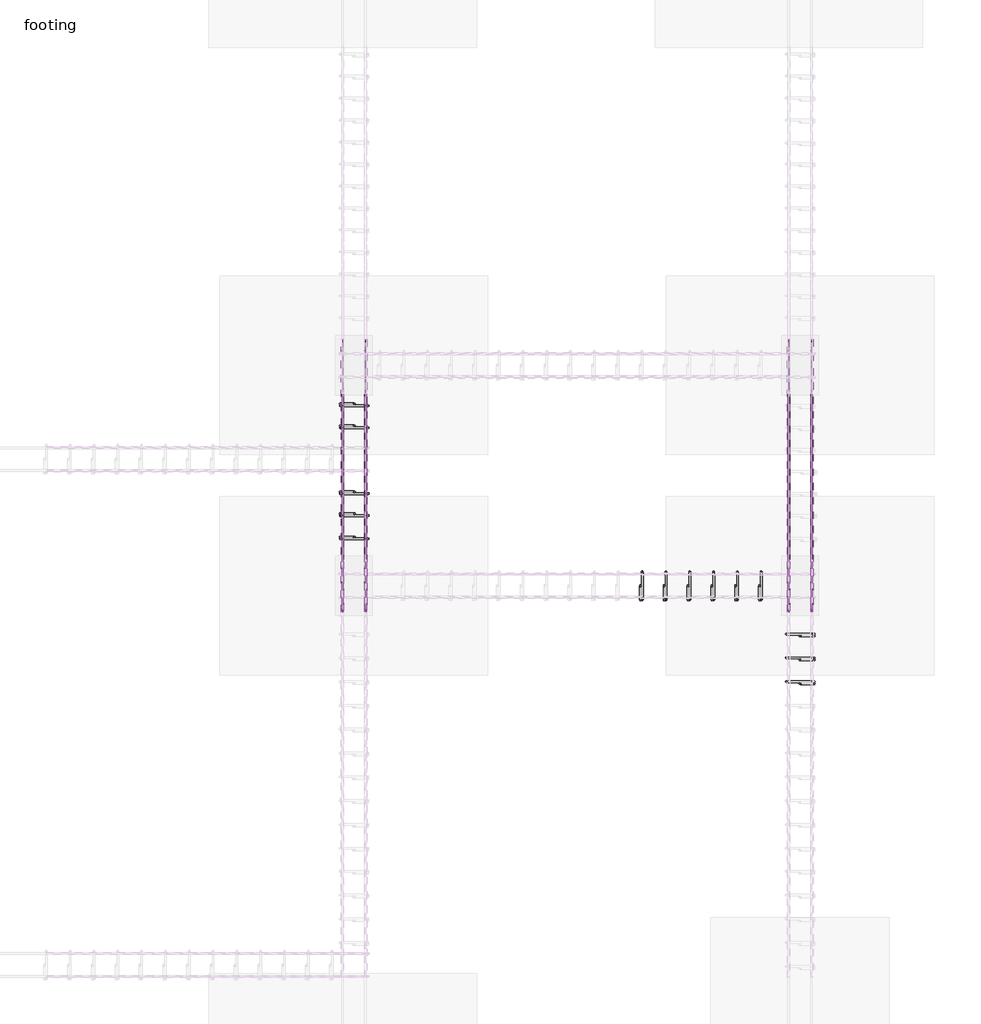
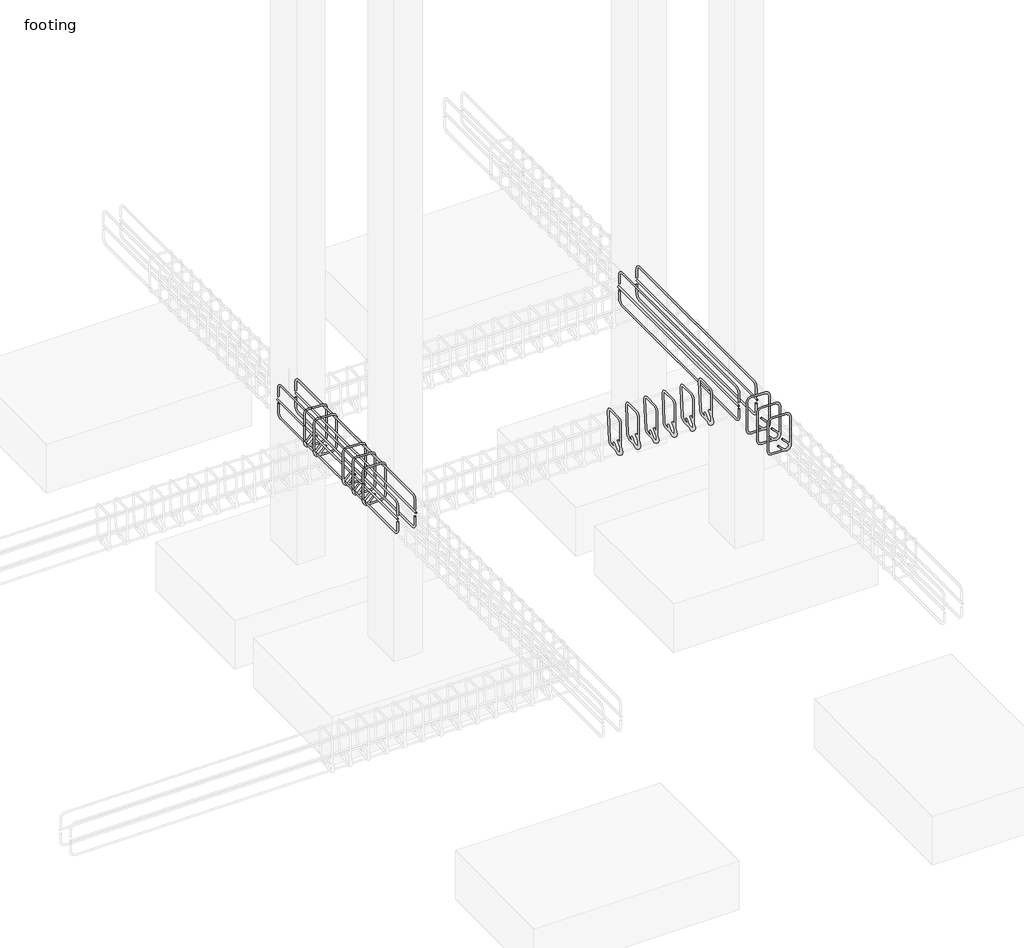
# One storey, part 14 of 21: 26 reinforcing bars.
"""IFC4 building model written with IfcOpenShell, lengths in millimetres."""

from ifc_helpers import new_model, si_unit, point, frame, origin, place, context, project, spatial, polyline, circle_curve, trimmed, segment, composite_curve, element, save
from ifc_brep_helpers import swept_disk

model = new_model("IFC4")

# Units and contexts
model_context = context("Model", 3, world=origin())
ifc_project = project(units=[si_unit("LENGTHUNIT", "METRE", prefix="MILLI")], contexts=[model_context])

# Site, building, storey
site = spatial("IfcSite", under=ifc_project)
building = spatial("IfcBuilding", under=site)
storey = spatial("IfcBuildingStorey", under=building, Name="footing", Elevation=-1524.0)

# Reinforcing bars
placement = place(None, origin())
element("IfcReinforcingBar", 1, at=placement, inside=storey, context=model_context, shape_type="SolidModel", body=[
    swept_disk(composite_curve([segment(polyline([(-5910.0883428, 6708.6887132, -310.8825168), (-5910.0883428, 6653.8237147, -365.7475153)]), True, "CONTINUOUS"), segment(trimmed(circle_curve(frame((-5910.0883428, 6631.3730744, -343.296875), z_axis=(-1.0, 0.0, 0.0), x_axis=(0.0, 22.450640299999577, -22.450640299999975)), 31.75), [point((-5910.0883428, 6653.8237147, -365.7475153))], [point((-5910.0883428, 6599.6230744, -343.296875))], True, "CARTESIAN"), True, "CONTINUOUS"), segment(polyline([(-5910.0883428, 6599.6230744, -343.296875), (-5910.0883428, 6599.6230744, -63.103125)]), True, "CONTINUOUS"), segment(trimmed(circle_curve(frame((-5910.0883428, 6631.3730744, -63.103125), z_axis=(-1.0, 0.0, 0.0), x_axis=(0.0, -31.75, 0.0)), 31.75), [point((-5910.0883428, 6599.6230744, -63.103125))], [point((-5910.0883428, 6631.3730744, -31.353125))], True, "CARTESIAN"), True, "CONTINUOUS"), segment(polyline([(-5910.0883428, 6631.3730744, -31.353125), (-5910.0883428, 6759.1668244, -31.353125)]), True, "CONTINUOUS"), segment(trimmed(circle_curve(frame((-5908.9159328, 6759.1668244, -63.0814712), z_axis=(-0.9993179916193466, 0.0, -0.03692629992126919), x_axis=(-1.1724100000001272, 0.0, 31.728346200000004)), 31.75), [point((-5910.0883428, 6759.1668244, -31.353125))], [point((-5908.9159328, 6790.9168244, -63.0814712))], True, "CARTESIAN"), True, "CONTINUOUS"), segment(polyline([(-5908.9159328, 6790.9168244, -63.0814712), (-5898.5607528, 6790.9168244, -343.3185288)]), True, "CONTINUOUS"), segment(trimmed(circle_curve(frame((-5898.5607528, 6759.1668244, -343.3185288), z_axis=(-0.9993179916193466, 0.0, -0.03692629992126919), x_axis=(0.0, 31.75, 0.0)), 31.75), [point((-5898.5607528, 6790.9168244, -343.3185288))], [point((-5897.3883428, 6759.1668244, -375.046875))], True, "CARTESIAN"), True, "CONTINUOUS"), segment(polyline([(-5897.3883428, 6759.1668244, -375.046875), (-5897.3883428, 6631.3730744, -375.046875)]), True, "CONTINUOUS"), segment(trimmed(circle_curve(frame((-5897.3883428, 6631.3730744, -343.296875), z_axis=(-1.0, 0.0, 0.0), x_axis=(0.0, 0.0, -31.75)), 31.75), [point((-5897.3883428, 6631.3730744, -375.046875))], [point((-5897.3883428, 6608.9224341, -320.8462347))], True, "CARTESIAN"), True, "CONTINUOUS"), segment(polyline([(-5897.3883428, 6608.9224341, -320.8462347), (-5897.3883428, 6663.7874326, -265.9812362)]), True, "CONTINUOUS")], self_intersect=False), 6.35),
])
element("IfcReinforcingBar", 2, at=placement, inside=storey, context=model_context, shape_type="SolidModel", body=[
    swept_disk(composite_curve([segment(polyline([(-5747.3883428, 6708.6887132, -310.8825168), (-5747.3883428, 6653.8237147, -365.7475153)]), True, "CONTINUOUS"), segment(trimmed(circle_curve(frame((-5747.3883428, 6631.3730744, -343.296875), z_axis=(-1.0, 0.0, 0.0), x_axis=(0.0, 22.450640299999577, -22.450640299999975)), 31.75), [point((-5747.3883428, 6653.8237147, -365.7475153))], [point((-5747.3883428, 6599.6230744, -343.296875))], True, "CARTESIAN"), True, "CONTINUOUS"), segment(polyline([(-5747.3883428, 6599.6230744, -343.296875), (-5747.3883428, 6599.6230744, -63.103125)]), True, "CONTINUOUS"), segment(trimmed(circle_curve(frame((-5747.3883428, 6631.3730744, -63.103125), z_axis=(-1.0, 0.0, 0.0), x_axis=(0.0, -31.75, 0.0)), 31.75), [point((-5747.3883428, 6599.6230744, -63.103125))], [point((-5747.3883428, 6631.3730744, -31.353125))], True, "CARTESIAN"), True, "CONTINUOUS"), segment(polyline([(-5747.3883428, 6631.3730744, -31.353125), (-5747.3883428, 6759.1668244, -31.353125)]), True, "CONTINUOUS"), segment(trimmed(circle_curve(frame((-5746.2159328, 6759.1668244, -63.0814712), z_axis=(-0.9993179916193466, 0.0, -0.03692629992126919), x_axis=(-1.1724100000001272, 0.0, 31.728346200000004)), 31.75), [point((-5747.3883428, 6759.1668244, -31.353125))], [point((-5746.2159328, 6790.9168244, -63.0814712))], True, "CARTESIAN"), True, "CONTINUOUS"), segment(polyline([(-5746.2159328, 6790.9168244, -63.0814712), (-5735.8607528, 6790.9168244, -343.3185288)]), True, "CONTINUOUS"), segment(trimmed(circle_curve(frame((-5735.8607528, 6759.1668244, -343.3185288), z_axis=(-0.9993179916193466, 0.0, -0.03692629992126919), x_axis=(0.0, 31.75, 0.0)), 31.75), [point((-5735.8607528, 6790.9168244, -343.3185288))], [point((-5734.6883428, 6759.1668244, -375.046875))], True, "CARTESIAN"), True, "CONTINUOUS"), segment(polyline([(-5734.6883428, 6759.1668244, -375.046875), (-5734.6883428, 6631.3730744, -375.046875)]), True, "CONTINUOUS"), segment(trimmed(circle_curve(frame((-5734.6883428, 6631.3730744, -343.296875), z_axis=(-1.0, 0.0, 0.0), x_axis=(0.0, 0.0, -31.75)), 31.75), [point((-5734.6883428, 6631.3730744, -375.046875))], [point((-5734.6883428, 6608.9224341, -320.8462347))], True, "CARTESIAN"), True, "CONTINUOUS"), segment(polyline([(-5734.6883428, 6608.9224341, -320.8462347), (-5734.6883428, 6663.7874326, -265.9812362)]), True, "CONTINUOUS")], self_intersect=False), 6.35),
])
element("IfcReinforcingBar", 3, at=placement, inside=storey, context=model_context, shape_type="SolidModel", body=[
    swept_disk(composite_curve([segment(polyline([(-5584.6883428, 6708.6887132, -310.8825168), (-5584.6883428, 6653.8237147, -365.7475153)]), True, "CONTINUOUS"), segment(trimmed(circle_curve(frame((-5584.6883428, 6631.3730744, -343.296875), z_axis=(-1.0, 0.0, 0.0), x_axis=(0.0, 22.450640299999577, -22.450640299999975)), 31.75), [point((-5584.6883428, 6653.8237147, -365.7475153))], [point((-5584.6883428, 6599.6230744, -343.296875))], True, "CARTESIAN"), True, "CONTINUOUS"), segment(polyline([(-5584.6883428, 6599.6230744, -343.296875), (-5584.6883428, 6599.6230744, -63.103125)]), True, "CONTINUOUS"), segment(trimmed(circle_curve(frame((-5584.6883428, 6631.3730744, -63.103125), z_axis=(-1.0, 0.0, 0.0), x_axis=(0.0, -31.75, 0.0)), 31.75), [point((-5584.6883428, 6599.6230744, -63.103125))], [point((-5584.6883428, 6631.3730744, -31.353125))], True, "CARTESIAN"), True, "CONTINUOUS"), segment(polyline([(-5584.6883428, 6631.3730744, -31.353125), (-5584.6883428, 6759.1668244, -31.353125)]), True, "CONTINUOUS"), segment(trimmed(circle_curve(frame((-5583.5159328, 6759.1668244, -63.0814712), z_axis=(-0.9993179916193466, 0.0, -0.03692629992126919), x_axis=(-1.1724100000001272, 0.0, 31.728346200000004)), 31.75), [point((-5584.6883428, 6759.1668244, -31.353125))], [point((-5583.5159328, 6790.9168244, -63.0814712))], True, "CARTESIAN"), True, "CONTINUOUS"), segment(polyline([(-5583.5159328, 6790.9168244, -63.0814712), (-5573.1607528, 6790.9168244, -343.3185288)]), True, "CONTINUOUS"), segment(trimmed(circle_curve(frame((-5573.1607528, 6759.1668244, -343.3185288), z_axis=(-0.9993179916193466, 0.0, -0.03692629992126919), x_axis=(0.0, 31.75, 0.0)), 31.75), [point((-5573.1607528, 6790.9168244, -343.3185288))], [point((-5571.9883428, 6759.1668244, -375.046875))], True, "CARTESIAN"), True, "CONTINUOUS"), segment(polyline([(-5571.9883428, 6759.1668244, -375.046875), (-5571.9883428, 6631.3730744, -375.046875)]), True, "CONTINUOUS"), segment(trimmed(circle_curve(frame((-5571.9883428, 6631.3730744, -343.296875), z_axis=(-1.0, 0.0, 0.0), x_axis=(0.0, 0.0, -31.75)), 31.75), [point((-5571.9883428, 6631.3730744, -375.046875))], [point((-5571.9883428, 6608.9224341, -320.8462347))], True, "CARTESIAN"), True, "CONTINUOUS"), segment(polyline([(-5571.9883428, 6608.9224341, -320.8462347), (-5571.9883428, 6663.7874326, -265.9812362)]), True, "CONTINUOUS")], self_intersect=False), 6.35),
])
element("IfcReinforcingBar", 4, at=placement, inside=storey, context=model_context, shape_type="SolidModel", body=[
    swept_disk(composite_curve([segment(polyline([(-5421.9883428, 6708.6887132, -310.8825168), (-5421.9883428, 6653.8237147, -365.7475153)]), True, "CONTINUOUS"), segment(trimmed(circle_curve(frame((-5421.9883428, 6631.3730744, -343.296875), z_axis=(-1.0, 0.0, 0.0), x_axis=(0.0, 22.450640299999577, -22.450640299999975)), 31.75), [point((-5421.9883428, 6653.8237147, -365.7475153))], [point((-5421.9883428, 6599.6230744, -343.296875))], True, "CARTESIAN"), True, "CONTINUOUS"), segment(polyline([(-5421.9883428, 6599.6230744, -343.296875), (-5421.9883428, 6599.6230744, -63.103125)]), True, "CONTINUOUS"), segment(trimmed(circle_curve(frame((-5421.9883428, 6631.3730744, -63.103125), z_axis=(-1.0, 0.0, 0.0), x_axis=(0.0, -31.75, 0.0)), 31.75), [point((-5421.9883428, 6599.6230744, -63.103125))], [point((-5421.9883428, 6631.3730744, -31.353125))], True, "CARTESIAN"), True, "CONTINUOUS"), segment(polyline([(-5421.9883428, 6631.3730744, -31.353125), (-5421.9883428, 6759.1668244, -31.353125)]), True, "CONTINUOUS"), segment(trimmed(circle_curve(frame((-5420.8159328, 6759.1668244, -63.0814712), z_axis=(-0.9993179916193466, 0.0, -0.03692629992126919), x_axis=(-1.1724100000001272, 0.0, 31.728346200000004)), 31.75), [point((-5421.9883428, 6759.1668244, -31.353125))], [point((-5420.8159328, 6790.9168244, -63.0814712))], True, "CARTESIAN"), True, "CONTINUOUS"), segment(polyline([(-5420.8159328, 6790.9168244, -63.0814712), (-5410.4607528, 6790.9168244, -343.3185288)]), True, "CONTINUOUS"), segment(trimmed(circle_curve(frame((-5410.4607528, 6759.1668244, -343.3185288), z_axis=(-0.9993179916193466, 0.0, -0.03692629992126919), x_axis=(0.0, 31.75, 0.0)), 31.75), [point((-5410.4607528, 6790.9168244, -343.3185288))], [point((-5409.2883428, 6759.1668244, -375.046875))], True, "CARTESIAN"), True, "CONTINUOUS"), segment(polyline([(-5409.2883428, 6759.1668244, -375.046875), (-5409.2883428, 6631.3730744, -375.046875)]), True, "CONTINUOUS"), segment(trimmed(circle_curve(frame((-5409.2883428, 6631.3730744, -343.296875), z_axis=(-1.0, 0.0, 0.0), x_axis=(0.0, 0.0, -31.75)), 31.75), [point((-5409.2883428, 6631.3730744, -375.046875))], [point((-5409.2883428, 6608.9224341, -320.8462347))], True, "CARTESIAN"), True, "CONTINUOUS"), segment(polyline([(-5409.2883428, 6608.9224341, -320.8462347), (-5409.2883428, 6663.7874326, -265.9812362)]), True, "CONTINUOUS")], self_intersect=False), 6.35),
])
element("IfcReinforcingBar", 5, at=placement, inside=storey, context=model_context, shape_type="SolidModel", body=[
    swept_disk(composite_curve([segment(polyline([(-5259.2883428, 6708.6887132, -310.8825168), (-5259.2883428, 6653.8237147, -365.7475153)]), True, "CONTINUOUS"), segment(trimmed(circle_curve(frame((-5259.2883428, 6631.3730744, -343.296875), z_axis=(-1.0, 0.0, 0.0), x_axis=(0.0, 22.450640299999577, -22.450640299999975)), 31.75), [point((-5259.2883428, 6653.8237147, -365.7475153))], [point((-5259.2883428, 6599.6230744, -343.296875))], True, "CARTESIAN"), True, "CONTINUOUS"), segment(polyline([(-5259.2883428, 6599.6230744, -343.296875), (-5259.2883428, 6599.6230744, -63.103125)]), True, "CONTINUOUS"), segment(trimmed(circle_curve(frame((-5259.2883428, 6631.3730744, -63.103125), z_axis=(-1.0, 0.0, 0.0), x_axis=(0.0, -31.75, 0.0)), 31.75), [point((-5259.2883428, 6599.6230744, -63.103125))], [point((-5259.2883428, 6631.3730744, -31.353125))], True, "CARTESIAN"), True, "CONTINUOUS"), segment(polyline([(-5259.2883428, 6631.3730744, -31.353125), (-5259.2883428, 6759.1668244, -31.353125)]), True, "CONTINUOUS"), segment(trimmed(circle_curve(frame((-5258.1159328, 6759.1668244, -63.0814712), z_axis=(-0.9993179916193466, 0.0, -0.03692629992126919), x_axis=(-1.1724099999992177, 0.0, 31.728346200000004)), 31.75), [point((-5259.2883428, 6759.1668244, -31.353125))], [point((-5258.1159328, 6790.9168244, -63.0814712))], True, "CARTESIAN"), True, "CONTINUOUS"), segment(polyline([(-5258.1159328, 6790.9168244, -63.0814712), (-5247.7607528, 6790.9168244, -343.3185288)]), True, "CONTINUOUS"), segment(trimmed(circle_curve(frame((-5247.7607528, 6759.1668244, -343.3185288), z_axis=(-0.9993179916193466, 0.0, -0.03692629992126919), x_axis=(0.0, 31.75, 0.0)), 31.75), [point((-5247.7607528, 6790.9168244, -343.3185288))], [point((-5246.5883428, 6759.1668244, -375.046875))], True, "CARTESIAN"), True, "CONTINUOUS"), segment(polyline([(-5246.5883428, 6759.1668244, -375.046875), (-5246.5883428, 6631.3730744, -375.046875)]), True, "CONTINUOUS"), segment(trimmed(circle_curve(frame((-5246.5883428, 6631.3730744, -343.296875), z_axis=(-1.0, 0.0, 0.0), x_axis=(0.0, 0.0, -31.75)), 31.75), [point((-5246.5883428, 6631.3730744, -375.046875))], [point((-5246.5883428, 6608.9224341, -320.8462347))], True, "CARTESIAN"), True, "CONTINUOUS"), segment(polyline([(-5246.5883428, 6608.9224341, -320.8462347), (-5246.5883428, 6663.7874326, -265.9812362)]), True, "CONTINUOUS")], self_intersect=False), 6.35),
])
element("IfcReinforcingBar", 6, at=placement, inside=storey, context=model_context, shape_type="SolidModel", body=[
    swept_disk(composite_curve([segment(polyline([(-5096.5883428, 6708.6887132, -310.8825168), (-5096.5883428, 6653.8237147, -365.7475153)]), True, "CONTINUOUS"), segment(trimmed(circle_curve(frame((-5096.5883428, 6631.3730744, -343.296875), z_axis=(-1.0, 0.0, 0.0), x_axis=(0.0, 22.450640299999577, -22.450640299999975)), 31.75), [point((-5096.5883428, 6653.8237147, -365.7475153))], [point((-5096.5883428, 6599.6230744, -343.296875))], True, "CARTESIAN"), True, "CONTINUOUS"), segment(polyline([(-5096.5883428, 6599.6230744, -343.296875), (-5096.5883428, 6599.6230744, -63.103125)]), True, "CONTINUOUS"), segment(trimmed(circle_curve(frame((-5096.5883428, 6631.3730744, -63.103125), z_axis=(-1.0, 0.0, 0.0), x_axis=(0.0, -31.75, 0.0)), 31.75), [point((-5096.5883428, 6599.6230744, -63.103125))], [point((-5096.5883428, 6631.3730744, -31.353125))], True, "CARTESIAN"), True, "CONTINUOUS"), segment(polyline([(-5096.5883428, 6631.3730744, -31.353125), (-5096.5883428, 6759.1668244, -31.353125)]), True, "CONTINUOUS"), segment(trimmed(circle_curve(frame((-5095.4159328, 6759.1668244, -63.0814712), z_axis=(-0.9993179916193466, 0.0, -0.03692629992126919), x_axis=(-1.1724100000001272, 0.0, 31.728346200000004)), 31.75), [point((-5096.5883428, 6759.1668244, -31.353125))], [point((-5095.4159328, 6790.9168244, -63.0814712))], True, "CARTESIAN"), True, "CONTINUOUS"), segment(polyline([(-5095.4159328, 6790.9168244, -63.0814712), (-5085.0607528, 6790.9168244, -343.3185288)]), True, "CONTINUOUS"), segment(trimmed(circle_curve(frame((-5085.0607528, 6759.1668244, -343.3185288), z_axis=(-0.9993179916193466, 0.0, -0.03692629992126919), x_axis=(0.0, 31.75, 0.0)), 31.75), [point((-5085.0607528, 6790.9168244, -343.3185288))], [point((-5083.8883428, 6759.1668244, -375.046875))], True, "CARTESIAN"), True, "CONTINUOUS"), segment(polyline([(-5083.8883428, 6759.1668244, -375.046875), (-5083.8883428, 6631.3730744, -375.046875)]), True, "CONTINUOUS"), segment(trimmed(circle_curve(frame((-5083.8883428, 6631.3730744, -343.296875), z_axis=(-1.0, 0.0, 0.0), x_axis=(0.0, 0.0, -31.75)), 31.75), [point((-5083.8883428, 6631.3730744, -375.046875))], [point((-5083.8883428, 6608.9224341, -320.8462347))], True, "CARTESIAN"), True, "CONTINUOUS"), segment(polyline([(-5083.8883428, 6608.9224341, -320.8462347), (-5083.8883428, 6663.7874326, -265.9812362)]), True, "CONTINUOUS")], self_intersect=False), 6.35),
])
element("IfcReinforcingBar", 7, at=placement, inside=storey, context=model_context, shape_type="SolidModel", body=[
    swept_disk(composite_curve([segment(polyline([(-7897.6815591, 7925.2699494, -265.9812362), (-7952.5465576, 7925.2699494, -320.8462347)]), True, "CONTINUOUS"), segment(trimmed(circle_curve(frame((-7930.0959173, 7925.2699494, -343.296875), z_axis=(0.0, -1.0, 0.0), x_axis=(-22.450640299999577, 0.0, 22.450640299999975)), 31.75), [point((-7952.5465576, 7925.2699494, -320.8462347))], [point((-7930.0959173, 7925.2699494, -375.046875))], True, "CARTESIAN"), True, "CONTINUOUS"), segment(polyline([(-7930.0959173, 7925.2699494, -375.046875), (-7802.3021673, 7925.2699494, -375.046875)]), True, "CONTINUOUS"), segment(trimmed(circle_curve(frame((-7802.3021673, 7925.2699494, -343.296875), z_axis=(0.0, -1.0, 0.0), x_axis=(0.0, 0.0, -31.75)), 31.75), [point((-7802.3021673, 7925.2699494, -375.046875))], [point((-7770.5521673, 7925.2699494, -343.296875))], True, "CARTESIAN"), True, "CONTINUOUS"), segment(polyline([(-7770.5521673, 7925.2699494, -343.296875), (-7770.5521673, 7925.2699494, -63.103125)]), True, "CONTINUOUS"), segment(trimmed(circle_curve(frame((-7802.2324265, 7927.3732031, -63.103125), z_axis=(-0.06624421176864148, -0.9978034397651431, 0.0), x_axis=(31.680259199999455, -2.1032537000000957, 0.0)), 31.75), [point((-7770.5521673, 7925.2699494, -63.103125))], [point((-7802.2324265, 7927.3732031, -31.353125))], True, "CARTESIAN"), True, "CONTINUOUS"), segment(polyline([(-7802.2324265, 7927.3732031, -31.353125), (-7930.165658, 7935.8666957, -31.353125)]), True, "CONTINUOUS"), segment(trimmed(circle_curve(frame((-7930.165658, 7935.8666957, -63.103125), z_axis=(-0.06624421176864148, -0.9978034397651431, 0.0), x_axis=(0.0, 0.0, 31.75)), 31.75), [point((-7930.165658, 7935.8666957, -31.353125))], [point((-7961.8459173, 7937.9699494, -63.103125))], True, "CARTESIAN"), True, "CONTINUOUS"), segment(polyline([(-7961.8459173, 7937.9699494, -63.103125), (-7961.8459173, 7937.9699494, -343.296875)]), True, "CONTINUOUS"), segment(trimmed(circle_curve(frame((-7930.0959173, 7937.9699494, -343.296875), z_axis=(0.0, -1.0, 0.0), x_axis=(-31.75, 0.0, 0.0)), 31.75), [point((-7961.8459173, 7937.9699494, -343.296875))], [point((-7907.645277, 7937.9699494, -365.7475153))], True, "CARTESIAN"), True, "CONTINUOUS"), segment(polyline([(-7907.645277, 7937.9699494, -365.7475153), (-7852.7802785, 7937.9699494, -310.8825168)]), True, "CONTINUOUS")], self_intersect=False), 6.35),
])
element("IfcReinforcingBar", 8, at=placement, inside=storey, context=model_context, shape_type="SolidModel", body=[
    swept_disk(composite_curve([segment(polyline([(-7943.5663014, 8372.0668244, -170.2827408), (-7943.5663014, 8372.0668244, -94.0827408)]), True, "CONTINUOUS"), segment(trimmed(circle_curve(frame((-7943.5663014, 8327.6168244, -94.0827408), z_axis=(1.0, 0.0, 0.0), x_axis=(0.0, 44.45000000000073, 0.0)), 44.45), [point((-7943.5663014, 8372.0668244, -94.0827408))], [point((-7943.5663014, 8327.6168244, -49.6327408))], True, "CARTESIAN"), True, "CONTINUOUS"), segment(polyline([(-7943.5663014, 8327.6168244, -49.6327408), (-7943.5663014, 6567.8730744, -49.6327408)]), True, "CONTINUOUS"), segment(trimmed(circle_curve(frame((-7943.5663014, 6567.8730744, -94.0827408), z_axis=(1.0, 0.0, 0.0), x_axis=(0.0, 0.0, 44.449999999999996)), 44.45), [point((-7943.5663014, 6567.8730744, -49.6327408))], [point((-7943.5663014, 6523.4230744, -94.0827408))], True, "CARTESIAN"), True, "CONTINUOUS"), segment(polyline([(-7943.5663014, 6523.4230744, -94.0827408), (-7943.5663014, 6523.4230744, -170.2827408)]), True, "CONTINUOUS")], self_intersect=False), 6.35),
])
element("IfcReinforcingBar", 9, at=placement, inside=storey, context=model_context, shape_type="SolidModel", body=[
    swept_disk(composite_curve([segment(polyline([(-7788.8317831, 8372.0668244, -170.2827408), (-7788.8317831, 8372.0668244, -94.0827408)]), True, "CONTINUOUS"), segment(trimmed(circle_curve(frame((-7788.8317831, 8327.6168244, -94.0827408), z_axis=(1.0, 0.0, 0.0), x_axis=(0.0, 44.45000000000073, 0.0)), 44.45), [point((-7788.8317831, 8372.0668244, -94.0827408))], [point((-7788.8317831, 8327.6168244, -49.6327408))], True, "CARTESIAN"), True, "CONTINUOUS"), segment(polyline([(-7788.8317831, 8327.6168244, -49.6327408), (-7788.8317831, 6567.8730744, -49.6327408)]), True, "CONTINUOUS"), segment(trimmed(circle_curve(frame((-7788.8317831, 6567.8730744, -94.0827408), z_axis=(1.0, 0.0, 0.0), x_axis=(0.0, 0.0, 44.449999999999996)), 44.45), [point((-7788.8317831, 6567.8730744, -49.6327408))], [point((-7788.8317831, 6523.4230744, -94.0827408))], True, "CARTESIAN"), True, "CONTINUOUS"), segment(polyline([(-7788.8317831, 6523.4230744, -94.0827408), (-7788.8317831, 6523.4230744, -170.2827408)]), True, "CONTINUOUS")], self_intersect=False), 6.35),
])
element("IfcReinforcingBar", 10, at=placement, inside=storey, context=model_context, shape_type="SolidModel", body=[
    swept_disk(composite_curve([segment(polyline([(-7943.5663014, 8372.0668244, -236.1172592), (-7943.5663014, 8372.0668244, -312.3172592)]), True, "CONTINUOUS"), segment(trimmed(circle_curve(frame((-7943.5663014, 8327.6168244, -312.3172592), z_axis=(-1.0, 0.0, 0.0), x_axis=(0.0, 44.45000000000073, 0.0)), 44.45), [point((-7943.5663014, 8372.0668244, -312.3172592))], [point((-7943.5663014, 8327.6168244, -356.7672592))], True, "CARTESIAN"), True, "CONTINUOUS"), segment(polyline([(-7943.5663014, 8327.6168244, -356.7672592), (-7943.5663014, 6567.8730744, -356.7672592)]), True, "CONTINUOUS"), segment(trimmed(circle_curve(frame((-7943.5663014, 6567.8730744, -312.3172592), z_axis=(-1.0, 0.0, 0.0), x_axis=(0.0, 0.0, -44.44999999999999)), 44.45), [point((-7943.5663014, 6567.8730744, -356.7672592))], [point((-7943.5663014, 6523.4230744, -312.3172592))], True, "CARTESIAN"), True, "CONTINUOUS"), segment(polyline([(-7943.5663014, 6523.4230744, -312.3172592), (-7943.5663014, 6523.4230744, -236.1172592)]), True, "CONTINUOUS")], self_intersect=False), 6.35),
])
element("IfcReinforcingBar", 11, at=placement, inside=storey, context=model_context, shape_type="SolidModel", body=[
    swept_disk(composite_curve([segment(polyline([(-7788.8317831, 8372.0668244, -236.1172592), (-7788.8317831, 8372.0668244, -312.3172592)]), True, "CONTINUOUS"), segment(trimmed(circle_curve(frame((-7788.8317831, 8327.6168244, -312.3172592), z_axis=(-1.0, 0.0, 0.0), x_axis=(0.0, 44.45000000000073, 0.0)), 44.45), [point((-7788.8317831, 8372.0668244, -312.3172592))], [point((-7788.8317831, 8327.6168244, -356.7672592))], True, "CARTESIAN"), True, "CONTINUOUS"), segment(polyline([(-7788.8317831, 8327.6168244, -356.7672592), (-7788.8317831, 6567.8730744, -356.7672592)]), True, "CONTINUOUS"), segment(trimmed(circle_curve(frame((-7788.8317831, 6567.8730744, -312.3172592), z_axis=(-1.0, 0.0, 0.0), x_axis=(0.0, 0.0, -44.44999999999999)), 44.45), [point((-7788.8317831, 6567.8730744, -356.7672592))], [point((-7788.8317831, 6523.4230744, -312.3172592))], True, "CARTESIAN"), True, "CONTINUOUS"), segment(polyline([(-7788.8317831, 6523.4230744, -312.3172592), (-7788.8317831, 6523.4230744, -236.1172592)]), True, "CONTINUOUS")], self_intersect=False), 6.35),
])
element("IfcReinforcingBar", 12, at=placement, inside=storey, context=model_context, shape_type="SolidModel", body=[
    swept_disk(composite_curve([segment(polyline([(-7949.1459173, 8378.4168244, -203.2), (-7949.1459173, 6517.0730744, -203.2)]), True, "CONTINUOUS")], self_intersect=False), 6.35),
])
element("IfcReinforcingBar", 13, at=placement, inside=storey, context=model_context, shape_type="SolidModel", body=[
    swept_disk(composite_curve([segment(polyline([(-7783.2521673, 8378.4168244, -203.2), (-7783.2521673, 6517.0730744, -203.2)]), True, "CONTINUOUS")], self_intersect=False), 6.35),
])
element("IfcReinforcingBar", 14, at=placement, inside=storey, context=model_context, shape_type="SolidModel", body=[
    swept_disk(composite_curve([segment(polyline([(-7897.6815591, 7775.2699494, -265.9812362), (-7952.5465576, 7775.2699494, -320.8462347)]), True, "CONTINUOUS"), segment(trimmed(circle_curve(frame((-7930.0959173, 7775.2699494, -343.296875), z_axis=(0.0, -1.0, 0.0), x_axis=(-22.450640299999577, 0.0, 22.450640299999975)), 31.75), [point((-7952.5465576, 7775.2699494, -320.8462347))], [point((-7930.0959173, 7775.2699494, -375.046875))], True, "CARTESIAN"), True, "CONTINUOUS"), segment(polyline([(-7930.0959173, 7775.2699494, -375.046875), (-7802.3021673, 7775.2699494, -375.046875)]), True, "CONTINUOUS"), segment(trimmed(circle_curve(frame((-7802.3021673, 7775.2699494, -343.296875), z_axis=(0.0, -1.0, 0.0), x_axis=(0.0, 0.0, -31.75)), 31.75), [point((-7802.3021673, 7775.2699494, -375.046875))], [point((-7770.5521673, 7775.2699494, -343.296875))], True, "CARTESIAN"), True, "CONTINUOUS"), segment(polyline([(-7770.5521673, 7775.2699494, -343.296875), (-7770.5521673, 7775.2699494, -63.103125)]), True, "CONTINUOUS"), segment(trimmed(circle_curve(frame((-7802.2324265, 7777.3732031, -63.103125), z_axis=(-0.06624421176864148, -0.9978034397651431, 0.0), x_axis=(31.680259199999455, -2.1032537000000957, 0.0)), 31.75), [point((-7770.5521673, 7775.2699494, -63.103125))], [point((-7802.2324265, 7777.3732031, -31.353125))], True, "CARTESIAN"), True, "CONTINUOUS"), segment(polyline([(-7802.2324265, 7777.3732031, -31.353125), (-7930.165658, 7785.8666957, -31.353125)]), True, "CONTINUOUS"), segment(trimmed(circle_curve(frame((-7930.165658, 7785.8666957, -63.103125), z_axis=(-0.06624421176864148, -0.9978034397651431, 0.0), x_axis=(0.0, 0.0, 31.75)), 31.75), [point((-7930.165658, 7785.8666957, -31.353125))], [point((-7961.8459173, 7787.9699494, -63.103125))], True, "CARTESIAN"), True, "CONTINUOUS"), segment(polyline([(-7961.8459173, 7787.9699494, -63.103125), (-7961.8459173, 7787.9699494, -343.296875)]), True, "CONTINUOUS"), segment(trimmed(circle_curve(frame((-7930.0959173, 7787.9699494, -343.296875), z_axis=(0.0, -1.0, 0.0), x_axis=(-31.75, 0.0, 0.0)), 31.75), [point((-7961.8459173, 7787.9699494, -343.296875))], [point((-7907.645277, 7787.9699494, -365.7475153))], True, "CARTESIAN"), True, "CONTINUOUS"), segment(polyline([(-7907.645277, 7787.9699494, -365.7475153), (-7852.7802785, 7787.9699494, -310.8825168)]), True, "CONTINUOUS")], self_intersect=False), 6.35),
])
element("IfcReinforcingBar", 15, at=placement, inside=storey, context=model_context, shape_type="SolidModel", body=[
    swept_disk(composite_curve([segment(polyline([(-7897.6815591, 7325.2699494, -265.9812362), (-7952.5465576, 7325.2699494, -320.8462347)]), True, "CONTINUOUS"), segment(trimmed(circle_curve(frame((-7930.0959173, 7325.2699494, -343.296875), z_axis=(0.0, -1.0, 0.0), x_axis=(-22.450640299999577, 0.0, 22.450640299999975)), 31.75), [point((-7952.5465576, 7325.2699494, -320.8462347))], [point((-7930.0959173, 7325.2699494, -375.046875))], True, "CARTESIAN"), True, "CONTINUOUS"), segment(polyline([(-7930.0959173, 7325.2699494, -375.046875), (-7802.3021673, 7325.2699494, -375.046875)]), True, "CONTINUOUS"), segment(trimmed(circle_curve(frame((-7802.3021673, 7325.2699494, -343.296875), z_axis=(0.0, -1.0, 0.0), x_axis=(0.0, 0.0, -31.75)), 31.75), [point((-7802.3021673, 7325.2699494, -375.046875))], [point((-7770.5521673, 7325.2699494, -343.296875))], True, "CARTESIAN"), True, "CONTINUOUS"), segment(polyline([(-7770.5521673, 7325.2699494, -343.296875), (-7770.5521673, 7325.2699494, -63.103125)]), True, "CONTINUOUS"), segment(trimmed(circle_curve(frame((-7802.2324265, 7327.3732031, -63.103125), z_axis=(-0.06624421176864148, -0.9978034397651431, 0.0), x_axis=(31.680259199999455, -2.1032537000000957, 0.0)), 31.75), [point((-7770.5521673, 7325.2699494, -63.103125))], [point((-7802.2324265, 7327.3732031, -31.353125))], True, "CARTESIAN"), True, "CONTINUOUS"), segment(polyline([(-7802.2324265, 7327.3732031, -31.353125), (-7930.165658, 7335.8666957, -31.353125)]), True, "CONTINUOUS"), segment(trimmed(circle_curve(frame((-7930.165658, 7335.8666957, -63.103125), z_axis=(-0.06624421176864148, -0.9978034397651431, 0.0), x_axis=(0.0, 0.0, 31.75)), 31.75), [point((-7930.165658, 7335.8666957, -31.353125))], [point((-7961.8459173, 7337.9699494, -63.103125))], True, "CARTESIAN"), True, "CONTINUOUS"), segment(polyline([(-7961.8459173, 7337.9699494, -63.103125), (-7961.8459173, 7337.9699494, -343.296875)]), True, "CONTINUOUS"), segment(trimmed(circle_curve(frame((-7930.0959173, 7337.9699494, -343.296875), z_axis=(0.0, -1.0, 0.0), x_axis=(-31.75, 0.0, 0.0)), 31.75), [point((-7961.8459173, 7337.9699494, -343.296875))], [point((-7907.645277, 7337.9699494, -365.7475153))], True, "CARTESIAN"), True, "CONTINUOUS"), segment(polyline([(-7907.645277, 7337.9699494, -365.7475153), (-7852.7802785, 7337.9699494, -310.8825168)]), True, "CONTINUOUS")], self_intersect=False), 6.35),
])
element("IfcReinforcingBar", 16, at=placement, inside=storey, context=model_context, shape_type="SolidModel", body=[
    swept_disk(composite_curve([segment(polyline([(-7897.6815591, 7175.2699494, -265.9812362), (-7952.5465576, 7175.2699494, -320.8462347)]), True, "CONTINUOUS"), segment(trimmed(circle_curve(frame((-7930.0959173, 7175.2699494, -343.296875), z_axis=(0.0, -1.0, 0.0), x_axis=(-22.450640299999577, 0.0, 22.450640299999975)), 31.75), [point((-7952.5465576, 7175.2699494, -320.8462347))], [point((-7930.0959173, 7175.2699494, -375.046875))], True, "CARTESIAN"), True, "CONTINUOUS"), segment(polyline([(-7930.0959173, 7175.2699494, -375.046875), (-7802.3021673, 7175.2699494, -375.046875)]), True, "CONTINUOUS"), segment(trimmed(circle_curve(frame((-7802.3021673, 7175.2699494, -343.296875), z_axis=(0.0, -1.0, 0.0), x_axis=(0.0, 0.0, -31.75)), 31.75), [point((-7802.3021673, 7175.2699494, -375.046875))], [point((-7770.5521673, 7175.2699494, -343.296875))], True, "CARTESIAN"), True, "CONTINUOUS"), segment(polyline([(-7770.5521673, 7175.2699494, -343.296875), (-7770.5521673, 7175.2699494, -63.103125)]), True, "CONTINUOUS"), segment(trimmed(circle_curve(frame((-7802.2324265, 7177.3732031, -63.103125), z_axis=(-0.06624421176864148, -0.9978034397651431, 0.0), x_axis=(31.680259199999455, -2.1032537000000957, 0.0)), 31.75), [point((-7770.5521673, 7175.2699494, -63.103125))], [point((-7802.2324265, 7177.3732031, -31.353125))], True, "CARTESIAN"), True, "CONTINUOUS"), segment(polyline([(-7802.2324265, 7177.3732031, -31.353125), (-7930.165658, 7185.8666957, -31.353125)]), True, "CONTINUOUS"), segment(trimmed(circle_curve(frame((-7930.165658, 7185.8666957, -63.103125), z_axis=(-0.06624421176864148, -0.9978034397651431, 0.0), x_axis=(0.0, 0.0, 31.75)), 31.75), [point((-7930.165658, 7185.8666957, -31.353125))], [point((-7961.8459173, 7187.9699494, -63.103125))], True, "CARTESIAN"), True, "CONTINUOUS"), segment(polyline([(-7961.8459173, 7187.9699494, -63.103125), (-7961.8459173, 7187.9699494, -343.296875)]), True, "CONTINUOUS"), segment(trimmed(circle_curve(frame((-7930.0959173, 7187.9699494, -343.296875), z_axis=(0.0, -1.0, 0.0), x_axis=(-31.75, 0.0, 0.0)), 31.75), [point((-7961.8459173, 7187.9699494, -343.296875))], [point((-7907.645277, 7187.9699494, -365.7475153))], True, "CARTESIAN"), True, "CONTINUOUS"), segment(polyline([(-7907.645277, 7187.9699494, -365.7475153), (-7852.7802785, 7187.9699494, -310.8825168)]), True, "CONTINUOUS")], self_intersect=False), 6.35),
])
element("IfcReinforcingBar", 17, at=placement, inside=storey, context=model_context, shape_type="SolidModel", body=[
    swept_disk(composite_curve([segment(polyline([(-7897.6815591, 7016.6456073, -265.9812362), (-7952.5465576, 7016.6456073, -320.8462347)]), True, "CONTINUOUS"), segment(trimmed(circle_curve(frame((-7930.0959173, 7016.6456073, -343.296875), z_axis=(0.0, -1.0, 0.0), x_axis=(-22.450640299999577, 0.0, 22.450640299999975)), 31.75), [point((-7952.5465576, 7016.6456073, -320.8462347))], [point((-7930.0959173, 7016.6456073, -375.046875))], True, "CARTESIAN"), True, "CONTINUOUS"), segment(polyline([(-7930.0959173, 7016.6456073, -375.046875), (-7802.3021673, 7016.6456073, -375.046875)]), True, "CONTINUOUS"), segment(trimmed(circle_curve(frame((-7802.3021673, 7016.6456073, -343.296875), z_axis=(0.0, -1.0, 0.0), x_axis=(0.0, 0.0, -31.75)), 31.75), [point((-7802.3021673, 7016.6456073, -375.046875))], [point((-7770.5521673, 7016.6456073, -343.296875))], True, "CARTESIAN"), True, "CONTINUOUS"), segment(polyline([(-7770.5521673, 7016.6456073, -343.296875), (-7770.5521673, 7016.6456073, -63.103125)]), True, "CONTINUOUS"), segment(trimmed(circle_curve(frame((-7802.2324265, 7018.748861, -63.103125), z_axis=(-0.06624421176864148, -0.9978034397651431, 0.0), x_axis=(31.680259199999455, -2.1032537000000957, 0.0)), 31.75), [point((-7770.5521673, 7016.6456073, -63.103125))], [point((-7802.2324265, 7018.748861, -31.353125))], True, "CARTESIAN"), True, "CONTINUOUS"), segment(polyline([(-7802.2324265, 7018.748861, -31.353125), (-7930.165658, 7027.2423536, -31.353125)]), True, "CONTINUOUS"), segment(trimmed(circle_curve(frame((-7930.165658, 7027.2423536, -63.103125), z_axis=(-0.06624421176864148, -0.9978034397651431, 0.0), x_axis=(0.0, 0.0, 31.75)), 31.75), [point((-7930.165658, 7027.2423536, -31.353125))], [point((-7961.8459173, 7029.3456073, -63.103125))], True, "CARTESIAN"), True, "CONTINUOUS"), segment(polyline([(-7961.8459173, 7029.3456073, -63.103125), (-7961.8459173, 7029.3456073, -343.296875)]), True, "CONTINUOUS"), segment(trimmed(circle_curve(frame((-7930.0959173, 7029.3456073, -343.296875), z_axis=(0.0, -1.0, 0.0), x_axis=(-31.75, 0.0, 0.0)), 31.75), [point((-7961.8459173, 7029.3456073, -343.296875))], [point((-7907.645277, 7029.3456073, -365.7475153))], True, "CARTESIAN"), True, "CONTINUOUS"), segment(polyline([(-7907.645277, 7029.3456073, -365.7475153), (-7852.7802785, 7029.3456073, -310.8825168)]), True, "CONTINUOUS")], self_intersect=False), 6.35),
])
element("IfcReinforcingBar", 18, at=placement, inside=storey, context=model_context, shape_type="SolidModel", body=[
    swept_disk(composite_curve([segment(polyline([(-4786.7165254, 6040.4456073, -265.9812362), (-4731.851527, 6040.4456073, -320.8462347)]), True, "CONTINUOUS"), segment(trimmed(circle_curve(frame((-4754.3021673, 6040.4456073, -343.296875), z_axis=(0.0, 1.0, 0.0), x_axis=(22.450640300000487, 0.0, 22.450640299999975)), 31.75), [point((-4731.851527, 6040.4456073, -320.8462347))], [point((-4754.3021673, 6040.4456073, -375.046875))], True, "CARTESIAN"), True, "CONTINUOUS"), segment(polyline([(-4754.3021673, 6040.4456073, -375.046875), (-4882.0959173, 6040.4456073, -375.046875)]), True, "CONTINUOUS"), segment(trimmed(circle_curve(frame((-4882.0959173, 6040.4456073, -343.296875), z_axis=(0.0, 1.0, 0.0), x_axis=(0.0, 0.0, -31.75)), 31.75), [point((-4882.0959173, 6040.4456073, -375.046875))], [point((-4913.8459173, 6040.4456073, -343.296875))], True, "CARTESIAN"), True, "CONTINUOUS"), segment(polyline([(-4913.8459173, 6040.4456073, -343.296875), (-4913.8459173, 6040.4456073, -63.103125)]), True, "CONTINUOUS"), segment(trimmed(circle_curve(frame((-4882.165658, 6038.3423536, -63.103125), z_axis=(0.0662442117686417, 0.9978034397651431, 0.0), x_axis=(-31.680259300000216, 2.1032537000000957, 0.0)), 31.75), [point((-4913.8459173, 6040.4456073, -63.103125))], [point((-4882.165658, 6038.3423536, -31.353125))], True, "CARTESIAN"), True, "CONTINUOUS"), segment(polyline([(-4882.165658, 6038.3423536, -31.353125), (-4754.2324265, 6029.848861, -31.353125)]), True, "CONTINUOUS"), segment(trimmed(circle_curve(frame((-4754.2324265, 6029.848861, -63.103125), z_axis=(0.06624421176864169, 0.997803439765143, 0.0), x_axis=(0.0, 0.0, 31.75)), 31.75), [point((-4754.2324265, 6029.848861, -31.353125))], [point((-4722.5521673, 6027.7456073, -63.103125))], True, "CARTESIAN"), True, "CONTINUOUS"), segment(polyline([(-4722.5521673, 6027.7456073, -63.103125), (-4722.5521673, 6027.7456073, -343.296875)]), True, "CONTINUOUS"), segment(trimmed(circle_curve(frame((-4754.3021673, 6027.7456073, -343.296875), z_axis=(0.0, 1.0, 0.0), x_axis=(31.75, 0.0, 0.0)), 31.75), [point((-4722.5521673, 6027.7456073, -343.296875))], [point((-4776.7528076, 6027.7456073, -365.7475153))], True, "CARTESIAN"), True, "CONTINUOUS"), segment(polyline([(-4776.7528076, 6027.7456073, -365.7475153), (-4831.617806, 6027.7456073, -310.8825168)]), True, "CONTINUOUS")], self_intersect=False), 6.35),
])
element("IfcReinforcingBar", 19, at=placement, inside=storey, context=model_context, shape_type="SolidModel", body=[
    swept_disk(composite_curve([segment(polyline([(-4786.7165254, 6203.1456073, -265.9812362), (-4731.851527, 6203.1456073, -320.8462347)]), True, "CONTINUOUS"), segment(trimmed(circle_curve(frame((-4754.3021673, 6203.1456073, -343.296875), z_axis=(0.0, 1.0, 0.0), x_axis=(22.450640300000487, 0.0, 22.450640299999975)), 31.75), [point((-4731.851527, 6203.1456073, -320.8462347))], [point((-4754.3021673, 6203.1456073, -375.046875))], True, "CARTESIAN"), True, "CONTINUOUS"), segment(polyline([(-4754.3021673, 6203.1456073, -375.046875), (-4882.0959173, 6203.1456073, -375.046875)]), True, "CONTINUOUS"), segment(trimmed(circle_curve(frame((-4882.0959173, 6203.1456073, -343.296875), z_axis=(0.0, 1.0, 0.0), x_axis=(0.0, 0.0, -31.75)), 31.75), [point((-4882.0959173, 6203.1456073, -375.046875))], [point((-4913.8459173, 6203.1456073, -343.296875))], True, "CARTESIAN"), True, "CONTINUOUS"), segment(polyline([(-4913.8459173, 6203.1456073, -343.296875), (-4913.8459173, 6203.1456073, -63.103125)]), True, "CONTINUOUS"), segment(trimmed(circle_curve(frame((-4882.165658, 6201.0423536, -63.103125), z_axis=(0.0662442117686417, 0.9978034397651431, 0.0), x_axis=(-31.680259300000216, 2.1032537000000957, 0.0)), 31.75), [point((-4913.8459173, 6203.1456073, -63.103125))], [point((-4882.165658, 6201.0423536, -31.353125))], True, "CARTESIAN"), True, "CONTINUOUS"), segment(polyline([(-4882.165658, 6201.0423536, -31.353125), (-4754.2324265, 6192.548861, -31.353125)]), True, "CONTINUOUS"), segment(trimmed(circle_curve(frame((-4754.2324265, 6192.548861, -63.103125), z_axis=(0.06624421176864169, 0.997803439765143, 0.0), x_axis=(0.0, 0.0, 31.75)), 31.75), [point((-4754.2324265, 6192.548861, -31.353125))], [point((-4722.5521673, 6190.4456073, -63.103125))], True, "CARTESIAN"), True, "CONTINUOUS"), segment(polyline([(-4722.5521673, 6190.4456073, -63.103125), (-4722.5521673, 6190.4456073, -343.296875)]), True, "CONTINUOUS"), segment(trimmed(circle_curve(frame((-4754.3021673, 6190.4456073, -343.296875), z_axis=(0.0, 1.0, 0.0), x_axis=(31.75, 0.0, 0.0)), 31.75), [point((-4722.5521673, 6190.4456073, -343.296875))], [point((-4776.7528076, 6190.4456073, -365.7475153))], True, "CARTESIAN"), True, "CONTINUOUS"), segment(polyline([(-4776.7528076, 6190.4456073, -365.7475153), (-4831.617806, 6190.4456073, -310.8825168)]), True, "CONTINUOUS")], self_intersect=False), 6.35),
])
element("IfcReinforcingBar", 20, at=placement, inside=storey, context=model_context, shape_type="SolidModel", body=[
    swept_disk(composite_curve([segment(polyline([(-4786.7165254, 6365.8456073, -265.9812362), (-4731.851527, 6365.8456073, -320.8462347)]), True, "CONTINUOUS"), segment(trimmed(circle_curve(frame((-4754.3021673, 6365.8456073, -343.296875), z_axis=(0.0, 1.0, 0.0), x_axis=(22.450640300000487, 0.0, 22.450640299999975)), 31.75), [point((-4731.851527, 6365.8456073, -320.8462347))], [point((-4754.3021673, 6365.8456073, -375.046875))], True, "CARTESIAN"), True, "CONTINUOUS"), segment(polyline([(-4754.3021673, 6365.8456073, -375.046875), (-4882.0959173, 6365.8456073, -375.046875)]), True, "CONTINUOUS"), segment(trimmed(circle_curve(frame((-4882.0959173, 6365.8456073, -343.296875), z_axis=(0.0, 1.0, 0.0), x_axis=(0.0, 0.0, -31.75)), 31.75), [point((-4882.0959173, 6365.8456073, -375.046875))], [point((-4913.8459173, 6365.8456073, -343.296875))], True, "CARTESIAN"), True, "CONTINUOUS"), segment(polyline([(-4913.8459173, 6365.8456073, -343.296875), (-4913.8459173, 6365.8456073, -63.103125)]), True, "CONTINUOUS"), segment(trimmed(circle_curve(frame((-4882.165658, 6363.7423536, -63.103125), z_axis=(0.0662442117686417, 0.9978034397651431, 0.0), x_axis=(-31.680259300000216, 2.1032537000000957, 0.0)), 31.75), [point((-4913.8459173, 6365.8456073, -63.103125))], [point((-4882.165658, 6363.7423536, -31.353125))], True, "CARTESIAN"), True, "CONTINUOUS"), segment(polyline([(-4882.165658, 6363.7423536, -31.353125), (-4754.2324265, 6355.248861, -31.353125)]), True, "CONTINUOUS"), segment(trimmed(circle_curve(frame((-4754.2324265, 6355.248861, -63.103125), z_axis=(0.06624421176864169, 0.997803439765143, 0.0), x_axis=(0.0, 0.0, 31.75)), 31.75), [point((-4754.2324265, 6355.248861, -31.353125))], [point((-4722.5521673, 6353.1456073, -63.103125))], True, "CARTESIAN"), True, "CONTINUOUS"), segment(polyline([(-4722.5521673, 6353.1456073, -63.103125), (-4722.5521673, 6353.1456073, -343.296875)]), True, "CONTINUOUS"), segment(trimmed(circle_curve(frame((-4754.3021673, 6353.1456073, -343.296875), z_axis=(0.0, 1.0, 0.0), x_axis=(31.75, 0.0, 0.0)), 31.75), [point((-4722.5521673, 6353.1456073, -343.296875))], [point((-4776.7528076, 6353.1456073, -365.7475153))], True, "CARTESIAN"), True, "CONTINUOUS"), segment(polyline([(-4776.7528076, 6353.1456073, -365.7475153), (-4831.617806, 6353.1456073, -310.8825168)]), True, "CONTINUOUS")], self_intersect=False), 6.35),
])
element("IfcReinforcingBar", 21, at=placement, inside=storey, context=model_context, shape_type="SolidModel", body=[
    swept_disk(composite_curve([segment(polyline([(-4895.5663014, 8372.0668244, -170.2827408), (-4895.5663014, 8372.0668244, -94.0827408)]), True, "CONTINUOUS"), segment(trimmed(circle_curve(frame((-4895.5663014, 8327.6168244, -94.0827408), z_axis=(1.0, 0.0, 0.0), x_axis=(0.0, 44.45000000000073, 0.0)), 44.45), [point((-4895.5663014, 8372.0668244, -94.0827408))], [point((-4895.5663014, 8327.6168244, -49.6327408))], True, "CARTESIAN"), True, "CONTINUOUS"), segment(polyline([(-4895.5663014, 8327.6168244, -49.6327408), (-4895.5663014, 6567.8730744, -49.6327408)]), True, "CONTINUOUS"), segment(trimmed(circle_curve(frame((-4895.5663014, 6567.8730744, -94.0827408), z_axis=(1.0, 0.0, 0.0), x_axis=(0.0, 0.0, 44.449999999999996)), 44.45), [point((-4895.5663014, 6567.8730744, -49.6327408))], [point((-4895.5663014, 6523.4230744, -94.0827408))], True, "CARTESIAN"), True, "CONTINUOUS"), segment(polyline([(-4895.5663014, 6523.4230744, -94.0827408), (-4895.5663014, 6523.4230744, -170.2827408)]), True, "CONTINUOUS")], self_intersect=False), 6.35),
])
element("IfcReinforcingBar", 22, at=placement, inside=storey, context=model_context, shape_type="SolidModel", body=[
    swept_disk(composite_curve([segment(polyline([(-4740.8317831, 8372.0668244, -170.2827408), (-4740.8317831, 8372.0668244, -94.0827408)]), True, "CONTINUOUS"), segment(trimmed(circle_curve(frame((-4740.8317831, 8327.6168244, -94.0827408), z_axis=(1.0, 0.0, 0.0), x_axis=(0.0, 44.45000000000073, 0.0)), 44.45), [point((-4740.8317831, 8372.0668244, -94.0827408))], [point((-4740.8317831, 8327.6168244, -49.6327408))], True, "CARTESIAN"), True, "CONTINUOUS"), segment(polyline([(-4740.8317831, 8327.6168244, -49.6327408), (-4740.8317831, 6567.8730744, -49.6327408)]), True, "CONTINUOUS"), segment(trimmed(circle_curve(frame((-4740.8317831, 6567.8730744, -94.0827408), z_axis=(1.0, 0.0, 0.0), x_axis=(0.0, 0.0, 44.449999999999996)), 44.45), [point((-4740.8317831, 6567.8730744, -49.6327408))], [point((-4740.8317831, 6523.4230744, -94.0827408))], True, "CARTESIAN"), True, "CONTINUOUS"), segment(polyline([(-4740.8317831, 6523.4230744, -94.0827408), (-4740.8317831, 6523.4230744, -170.2827408)]), True, "CONTINUOUS")], self_intersect=False), 6.35),
])
element("IfcReinforcingBar", 23, at=placement, inside=storey, context=model_context, shape_type="SolidModel", body=[
    swept_disk(composite_curve([segment(polyline([(-4895.5663014, 8372.0668244, -236.1172592), (-4895.5663014, 8372.0668244, -312.3172592)]), True, "CONTINUOUS"), segment(trimmed(circle_curve(frame((-4895.5663014, 8327.6168244, -312.3172592), z_axis=(-1.0, 0.0, 0.0), x_axis=(0.0, 44.45000000000073, 0.0)), 44.45), [point((-4895.5663014, 8372.0668244, -312.3172592))], [point((-4895.5663014, 8327.6168244, -356.7672592))], True, "CARTESIAN"), True, "CONTINUOUS"), segment(polyline([(-4895.5663014, 8327.6168244, -356.7672592), (-4895.5663014, 6567.8730744, -356.7672592)]), True, "CONTINUOUS"), segment(trimmed(circle_curve(frame((-4895.5663014, 6567.8730744, -312.3172592), z_axis=(-1.0, 0.0, 0.0), x_axis=(0.0, 0.0, -44.44999999999999)), 44.45), [point((-4895.5663014, 6567.8730744, -356.7672592))], [point((-4895.5663014, 6523.4230744, -312.3172592))], True, "CARTESIAN"), True, "CONTINUOUS"), segment(polyline([(-4895.5663014, 6523.4230744, -312.3172592), (-4895.5663014, 6523.4230744, -236.1172592)]), True, "CONTINUOUS")], self_intersect=False), 6.35),
])
element("IfcReinforcingBar", 24, at=placement, inside=storey, context=model_context, shape_type="SolidModel", body=[
    swept_disk(composite_curve([segment(polyline([(-4740.8317831, 8372.0668244, -236.1172592), (-4740.8317831, 8372.0668244, -312.3172592)]), True, "CONTINUOUS"), segment(trimmed(circle_curve(frame((-4740.8317831, 8327.6168244, -312.3172592), z_axis=(-1.0, 0.0, 0.0), x_axis=(0.0, 44.45000000000073, 0.0)), 44.45), [point((-4740.8317831, 8372.0668244, -312.3172592))], [point((-4740.8317831, 8327.6168244, -356.7672592))], True, "CARTESIAN"), True, "CONTINUOUS"), segment(polyline([(-4740.8317831, 8327.6168244, -356.7672592), (-4740.8317831, 6567.8730744, -356.7672592)]), True, "CONTINUOUS"), segment(trimmed(circle_curve(frame((-4740.8317831, 6567.8730744, -312.3172592), z_axis=(-1.0, 0.0, 0.0), x_axis=(0.0, 0.0, -44.44999999999999)), 44.45), [point((-4740.8317831, 6567.8730744, -356.7672592))], [point((-4740.8317831, 6523.4230744, -312.3172592))], True, "CARTESIAN"), True, "CONTINUOUS"), segment(polyline([(-4740.8317831, 6523.4230744, -312.3172592), (-4740.8317831, 6523.4230744, -236.1172592)]), True, "CONTINUOUS")], self_intersect=False), 6.35),
])
element("IfcReinforcingBar", 25, at=placement, inside=storey, context=model_context, shape_type="SolidModel", body=[
    swept_disk(composite_curve([segment(polyline([(-4901.1459173, 8378.4168244, -203.2), (-4901.1459173, 6517.0730744, -203.2)]), True, "CONTINUOUS")], self_intersect=False), 6.35),
])
element("IfcReinforcingBar", 26, at=placement, inside=storey, context=model_context, shape_type="SolidModel", body=[
    swept_disk(composite_curve([segment(polyline([(-4735.2521673, 8378.4168244, -203.2), (-4735.2521673, 6517.0730744, -203.2)]), True, "CONTINUOUS")], self_intersect=False), 6.35),
])

save(model, "model.ifc")

# Revit data of these elements
# Elements 1, 2, 3, 4, 5, 6, 7, 8, 9, 10, 11, 12, 13, 14, 15, 16, 17, 18, 19, 20, 21, 22, 23, 24, 25, 26 (IfcReinforcingBar)
#   Phase Created = New Construction
